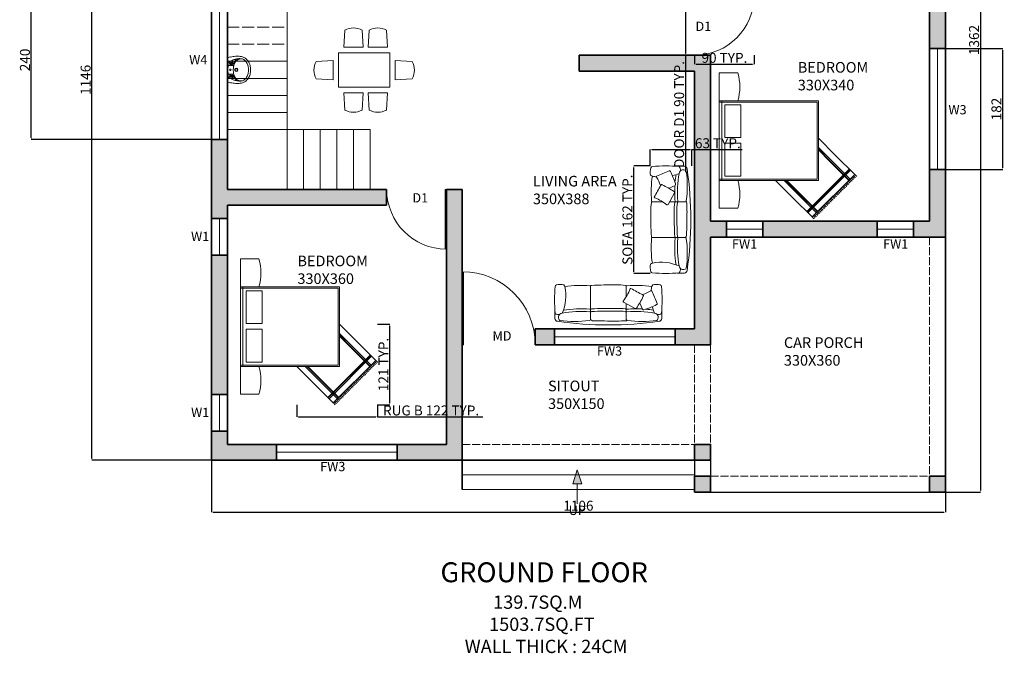
# Model space of a CAD drawing. Units: centimetres. Extents: x 2449 to 7478, y 778 to 2486.
# Tile 7 of 9: x 5994 to 7478, y 778 to 1732. Entities that reach past the tile are written whole.
import ezdxf

# ---------------------------------------------------------------- set-up
doc = ezdxf.new("R2010")
doc.units = ezdxf.units.CM
doc.linetypes.add('ACAD_ISO02W100', pattern=[15, 12, -3])
for name, color, linetype, lineweight in [('0.15', 34, 'Continuous', 15), ('A-ANNO-DIMS', 2, 'Continuous', 18), ('A-ANNO-SYMB', 8, 'Continuous', 18), ('A-ANNO-TEXT', 7, 'Continuous', 18), ('A-ANNO-TITL', 7, 'Continuous', 25), ('A-AREA-IDEN', 7, 'Continuous', 18), ('A-COLS', 7, 'Continuous', 35), ('A-COLS-PATT', 7, 'Continuous', 13), ('A-DOOR', 4, 'Continuous', 18), ('A-FLOR', 7, 'Continuous', 25), ('A-FLOR-FIXT', 8, 'Continuous', 18), ('A-FLOR-OVHD', 8, 'ACAD_ISO02W100', 18), ('A-FLOR-STRS', 7, 'Continuous', 18), ('A-FLOR-STRS-OVHD', 7, 'ACAD_ISO02W100', 13), ('A-WALL', 7, 'Continuous', 35), ('A-WALL-PATT', 7, 'Continuous', 13), ('B-FURNITURE', 22, 'Continuous', 18), ('Win', 1, 'Continuous', 18)]:
    doc.layers.add(name, color=color, linetype=linetype, lineweight=lineweight)
doc.styles.get("Standard").update_dxf_attribs({"font": 'arial.ttf'})
doc.dimstyles.new('ISO-25', dxfattribs={"dimtxt": 15, "dimasz": 2.5, "dimexe": 0, "dimexo": 0, "dimgap": 0, "dimtad": 1, "dimtxsty": 'Standard', "dimcen": 2.5, "dimadec": 0, "dimazin": 0, "dimtfac": 1, "dimtmove": 0, "dimatfit": 3, "dimfxl": 1, "dimarcsym": 0})

# ---------------------------------------------------------------- blocks, each defined once
blk = doc.blocks.new('ролар')
at = {"layer": 'B-FURNITURE'}
for p, q in [((182149, -12928), (182149, -13090)), ((182946, -12908), (182946, -13070)), ((183742, -12908), (183742, -13070)), ((184538, -12927), (184538, -13090)), ((182946, -13070), (182946, -13655)), ((183742, -13070), (183742, -13261)), ((183742, -13412), (183742, -13655))]:
    blk.add_line(p, q, dxfattribs=at)
blk.add_lwpolyline([(184124, -13426, 0.039108), (183972, -13160, 0.352413), (183942, -13151), (183685, -13293, 0.370087), (183675, -13320, -0.085318), (183831, -13592, 0.338149), (183848, -13604, -0.006963), (184118, -13456, 0.478074)], format="xyb", close=True, dxfattribs=at)
blk.add_lwpolyline([(184112, -13464, -0.054969), (184295, -13552, 0.338149), (184316, -13550, -0.006963), (184437, -13268, 0.478074), (184423, -13240, 0.039108), (184140, -13125, 0.352413), (184110, -13136), (184052, -13272)], format="xyb", dxfattribs=at)
for centre, radius, start, end in [((182209, -12928), 60, 90, 180), ((183344, -20690), 7904, 81.7476, 98.2524), ((182322, -12954), 95.7, 154.4132, 226.8965), ((182264, -12914), 28.1, 104.7154, 176.7534), ((182585, -15161), 2298, 81.7903, 98.2097), ((182918, -12915), 28.9, 15.2961, 99.1888), ((182999, -12942), 63.3, 99.7658, 147.0241), ((181568, 80195), 93085, 270.87421, 271.20678), ((183296, -20822), 7955, 86.6979, 88.3256), ((183770, -12915), 28.9, 80.8112, 164.7039), ((184102, -15161), 2298, 81.7903, 98.2097), ((184423, -12914), 28.1, 3.2466, 75.2846), ((184365, -12954), 95.7, 313.1035, 25.5868), ((184478, -12928), 60, 358.6006, 89.9879), ((186046, -13346), 3905, 175.5762, 184.4238), ((182224, -13128), 110, 72.3508, 130.321), ((182340, -12922), 131, 230.7956, 255.727), ((181452, -13440), 941, 347.608, 24.5904), ((182727, -10699), 2387, 259.8888, 274.8671), ((182725, -10712), 2434, 260.7796, 274.8194), ((182927, -13057), 20.3, 275.8765, 1.8), ((182927, -13117), 20.3, 275.8765, 1.8), ((182962, -13065), 17.3, 149.88, 272.0041), ((182962, -13125), 17.3, 149.88, 272.0041), ((183401, -6361), 6736, 266.2761, 271.089), ((183401, -6421), 6736, 266.2761, 271.089), ((183573, -12278), 819, 266.8813, 280.6931), ((183573, -12338), 819, 266.8813, 280.6931), ((183725, -13065), 17.3, 267.9959, 30.12), ((183725, -13125), 17.3, 267.9959, 30.12), ((183760, -13057), 20.3, 178.2, 264.1235), ((183760, -13117), 20.3, 178.2, 264.1235), ((183961, -10699), 2387, 265.1329, 280.1112), ((184001, -9721), 3425, 265.9379, 271.7664), ((184034, -11509), 1637, 275.2593, 281.2487), ((185235, -13440), 941, 155.4096, 164.8885), ((184348, -12922), 131, 284.273, 309.2044), ((184464, -13128), 110, 49.679, 107.6492), ((180641, -13346), 3905, 355.5762, 4.4238), ((182195, -13642), 42.7, 187.075, 250.1971), ((181903, -13435), 512, 330.8359, 336.0732), ((182722, -11168), 2503, 261.8987, 274.7524), ((182927, -13643), 20.3, 275.8765, 1.8), ((182962, -13651), 17.3, 149.88, 272.0041), ((183725, -13651), 17.3, 267.9959, 30.12), ((183760, -13643), 20.3, 178.2, 264.1235), ((183966, -11168), 2503, 265.2476, 278.1013), ((185235, -13440), 941, 186.9661, 192.392), ((184785, -13435), 512, 203.9268, 209.1641), ((184493, -13642), 42.7, 289.8029, 352.925), ((182270, -13358), 336, 254.5718, 283.8571), ((183401, -6946), 6736, 266.2761, 271.089), ((183573, -12863), 819, 266.8813, 280.6931), ((184418, -13358), 336, 256.1429, 285.4282)]:
    blk.add_arc(centre, radius, start, end, dxfattribs=at)
blk = doc.blocks.new('table-11')
at = {"color": 0, "linetype": 'ByBlock'}
for p, q in [((-1.122, 0.533), (-1.144, 0.134)), ((-0.716, 0.533), (-0.694, 0.134)), ((-0.554, 0.533), (-0.576, 0.134)), ((-0.148, 0.533), (-0.126, 0.134)), ((0, 0), (-1.2, 0)), ((-1.2, -0.8), (-1.2, 0)), ((-1.144, 0.134), (-0.694, 0.134)), ((-0.576, 0.134), (-0.126, 0.134)), ((0, -0.8), (0, 0)), ((-1.723, -0.197), (-1.324, -0.175)), ((-1.324, -0.625), (-1.324, -0.175)), ((0.523, -0.197), (0.124, -0.175)), ((0.124, -0.625), (0.124, -0.175)), ((-1.723, -0.603), (-1.324, -0.625)), ((0.523, -0.603), (0.124, -0.625)), ((0, -0.8), (-1.2, -0.8)), ((-1.144, -0.934), (-0.694, -0.934)), ((-1.122, -1.333), (-1.144, -0.934)), ((-0.716, -1.333), (-0.694, -0.934)), ((-0.576, -0.934), (-0.126, -0.934)), ((-0.554, -1.333), (-0.576, -0.934)), ((-0.148, -1.333), (-0.126, -0.934))]:
    blk.add_line(p, q, dxfattribs=at)
for centre, start, end in [((-0.919, 0.159), 61.4891, 118.5109), ((-0.351, 0.159), 61.4891, 118.5109), ((-1.349, -0.4), 151.4891, 208.5109), ((0.149, -0.4), 331.4891, 28.5109), ((-0.919, -0.959), 241.4891, 298.5109), ((-0.351, -0.959), 241.4891, 298.5109)]:
    blk.add_arc(centre, 0.425, start, end, dxfattribs=at)
blk = doc.blocks.new('A$C376C2187')
at = {"layer": 'B-FURNITURE'}
for p, q in [((-1.53, 1.82), (-1.53, 2.24)), ((-1.53, 2.24), (-0.9, 2.24)), ((-0.9, 0), (-0.9, 2.24)), ((-0.9, 2.24), (0.9, 2.24)), ((-0.9, 2.24), (-0.9, 1.82)), ((-0.87, 0.03), (-0.87, 2.24)), ((0.87, 2.24), (0.87, 0.03)), ((0.9, 2.24), (0.9, 0)), ((0.9, 1.82), (0.9, 2.24)), ((0.9, 2.24), (1.53, 2.24)), ((1.53, 2.24), (1.53, 1.82)), ((-0.9, 2.182), (0.9, 2.182)), ((-0.807, 2.112), (-0.057, 2.112)), ((-0.807, 1.749), (-0.807, 2.112)), ((-0.057, 2.112), (-0.057, 1.749)), ((0.069, 2.112), (0.807, 2.112)), ((0.069, 2.112), (0.069, 1.749)), ((0.807, 2.112), (0.807, 1.749)), ((-0.807, 1.749), (-0.057, 1.749)), ((0.069, 1.749), (0.807, 1.749)), ((0.9, 0), (-0.9, 0)), ((0.87, 0.03), (-0.87, 0.03))]:
    blk.add_line(p, q, dxfattribs=at)
for centre in [(-1.215, 2.926), (1.215, 2.926)]:
    blk.add_arc(centre, 1.15, 254.0965, 285.9035, dxfattribs=at)
blk = doc.blocks.new('lavamanos 2')
at = {"layer": '0.15'}
for p, q in [((0, 0.234), (0, -0.234)), ((-0.13, 0.11), (-0.131, 0.11)), ((-0.014, 0.087), (-0.13, 0.086)), ((-0.113, 0.112), (-0.107, 0.158)), ((-0.104, 0.111), (-0.098, 0.157)), ((-0.086, 0.109), (-0.081, 0.147)), ((-0.077, 0.107), (-0.072, 0.145)), ((-0.059, 0.105), (-0.055, 0.135)), ((-0.05, 0.104), (-0.046, 0.134)), ((-0.13, -0.11), (-0.131, -0.11)), ((-0.014, -0.087), (-0.13, -0.086)), ((-0.113, -0.112), (-0.107, -0.158)), ((-0.104, -0.111), (-0.098, -0.157)), ((-0.086, -0.109), (-0.081, -0.147)), ((-0.077, -0.107), (-0.072, -0.145)), ((-0.059, -0.105), (-0.055, -0.135)), ((-0.05, -0.104), (-0.046, -0.134))]:
    blk.add_line(p, q, dxfattribs=at)
for centre, radius in [((-0.178, 0), 0.035), ((-0.178, 0), 0.0235), ((-0.06, 0), 0.015)]:
    blk.add_circle(centre, radius, dxfattribs=at)
for centre, radius, start, end in [((-0.166, 0.001), 0.302, 136.5719, 154.3277), ((-0.242, 0.066), 0.202, 108.1945, 135.3686), ((-0.242, 0.065), 0.164, 121.9929, 150.5889), ((-0.266, 0.104), 0.119, 92.4774, 122.1411), ((-0.203, -0.086), 0.359, 91.203, 106.4255), ((-0.277, 0.068), 0.153, 57.2491, 95.54), ((-0.244, -0.013), 0.237, 77.2482, 96.4632), ((-0.221, -0.685), 0.959, 86.5514, 89.4131), ((-0.277, 0.068), 0.168, 56.8766, 64.9971), ((-0.222, 0.003), 0.218, 71.9849, 82.0124), ((-0.366, -0.002), 0.278, 40.3525, 49.2255), ((-0.212, -0.548), 0.82, 83.1224, 86.5796), ((-0.31, -0.315), 0.547, 69.5191, 73.4912), ((-0.299, -0.285), 0.516, 65.23, 69.5378), ((5.828, 30.215), 30.532, 258.7782, 258.876), ((-0.126, -0.066), 0.329, 69.0601, 78.8218), ((-0.02, 0.212), 0.0314, 54.7949, 69.0601), ((-0.005, 0.234), 0.005, 0, 54.7949), ((-0.209, 0.006), 0.256, 171.3102, 181.2627), ((-0.209, -0.006), 0.256, 178.7373, 188.6898), ((-0.056, -0.018), 0.411, 158.7011, 171.3102), ((0.466, -0.083), 0.895, 169.8632, 174.658), ((0.466, 0.083), 0.895, 185.342, 190.1368), ((-0.2, 0.026), 0.22, 147.1156, 167.4425), ((-0.366, -0.002), 0.263, 40.3525, 49.0046), ((-0.237, 0.11), 0.0921, 27.3186, 39.1156), ((-0.349, 0.036), 0.226, 22.3361, 30.8927), ((-0.237, 0.11), 0.107, 27.5743, 39.1156), ((-0.349, 0.036), 0.241, 22.1921, 30.7838), ((-1.266, -0.239), 1.182, 16.3631, 17.7767), ((-0.132, 0.117), 0.007, 197.4099, 270.4949), ((0.185, 0.165), 0.325, 192.5389, 196.7072), ((-0.13, 0.117), 0.007, 270.4949, 17.3953), ((-1.266, -0.239), 1.197, 17.3953, 17.8049), ((0.389, 0.121), 0.517, 185.5053, 189.8131), ((-0.718, -0.007), 0.599, 0.6765, 3.8216), ((-0.718, 0.007), 0.599, 356.1784, 359.3235), ((-0.108, 0.111), 0.0045, 172.614, 352.614), ((-0.102, 0.158), 0.0045, 352.614, 172.614), ((-0.081, 0.108), 0.0045, 172.614, 352.614), ((-0.278, -0.241), 0.466, 60.2413, 65.2382), ((-0.076, 0.146), 0.0045, 352.614, 172.614), ((-0.054, 0.104), 0.0045, 172.614, 352.614), ((-0.05, 0.135), 0.0045, 352.614, 172.614), ((-0.065, 0.118), 0.049, 1.5827, 68.6208), ((-2.148, 0.001), 2.135, 359.9754, 3.1901), ((-2.148, -0.001), 2.135, 356.8099, 0.0246), ((-0.056, 0.018), 0.411, 188.6898, 201.2989), ((-0.166, -0.001), 0.302, 205.6723, 223.4281), ((-0.2, -0.026), 0.22, 192.5575, 212.8844), ((-0.242, -0.065), 0.164, 209.4111, 238.0071), ((-0.277, -0.068), 0.153, 264.46, 302.7509), ((-0.366, 0.002), 0.263, 310.9954, 319.6475), ((-0.366, 0.002), 0.278, 310.7745, 319.6475), ((-0.237, -0.11), 0.0921, 320.8844, 332.6814), ((-0.349, -0.036), 0.226, 329.1073, 337.6639), ((-0.237, -0.11), 0.107, 320.8844, 332.4257), ((-0.349, -0.036), 0.241, 329.2162, 337.8079), ((-1.266, 0.239), 1.182, 342.2233, 343.6369), ((-0.132, -0.117), 0.007, 89.5051, 162.5901), ((0.185, -0.165), 0.325, 163.2928, 167.4611), ((-0.13, -0.117), 0.007, 342.6047, 89.5051), ((0.389, -0.121), 0.517, 170.1869, 174.4947), ((-1.266, 0.239), 1.197, 342.1951, 342.6047), ((-0.299, 0.286), 0.516, 290.4622, 294.77), ((-0.108, -0.111), 0.0045, 7.386, 187.386), ((-0.102, -0.158), 0.0045, 187.386, 7.386), ((-0.081, -0.108), 0.0045, 7.386, 187.386), ((-0.278, 0.241), 0.466, 294.7618, 299.7587), ((-0.076, -0.146), 0.0045, 187.386, 7.386), ((-0.054, -0.104), 0.0045, 7.386, 187.386), ((-0.05, -0.135), 0.0045, 187.386, 7.386), ((-0.065, -0.118), 0.049, 291.3792, 358.4173), ((-0.242, -0.066), 0.202, 224.6314, 251.8055), ((-0.266, -0.104), 0.119, 237.8589, 267.5226), ((-0.203, 0.086), 0.359, 253.5745, 268.797), ((-0.244, 0.013), 0.237, 263.5368, 282.7518), ((-0.221, 0.685), 0.959, 270.5869, 273.4486), ((-0.277, -0.068), 0.168, 295.0029, 303.1234), ((-0.222, -0.003), 0.218, 277.9876, 288.0151), ((-0.212, 0.548), 0.82, 273.4204, 276.8776), ((-0.31, 0.315), 0.547, 286.5088, 290.4809), ((5.828, -30.215), 30.532, 101.124, 101.2218), ((-0.126, 0.066), 0.329, 281.1782, 290.9399), ((-0.02, -0.212), 0.0314, 290.9399, 305.2051), ((-0.005, -0.234), 0.005, 305.2051, 0)]:
    blk.add_arc(centre, radius, start, end, dxfattribs=at)
blk = doc.blocks.new('1')
for p, q in [((5854.1, 1703.8), (5854.1, 1593.8)), ((5856.1, 1703.8), (5856.1, 1593.8)), ((5856.1, 1593.8), (5854.1, 1593.8))]:
    blk.add_line(p, q)
blk.add_arc((5854.1, 1593.8), 110, 0, 90)
blk = doc.blocks.new('2')
for p, q in [((5717.3, 1812.7), (5717.3, 1722.7)), ((5719.3, 1812.7), (5719.3, 1722.7)), ((5719.3, 1722.7), (5717.3, 1722.7))]:
    blk.add_line(p, q)
blk.add_arc((5717.3, 1722.7), 90, 0, 90)
blk = doc.blocks.new('*D64')
at = {"layer": 'A-ANNO-DIMS', "color": 0, "lineweight": -2, "transparency": 16777216}
for p, q in [((7389, 2382.3), (7441.8, 2382.3)), ((7441.8, 2379.8), (7441.8, 1022.8)), ((7389, 1020.3), (7441.8, 1020.3))]:
    blk.add_line(p, q, dxfattribs=at)
at = {"layer": 'A-ANNO-DIMS', "color": 0, "transparency": 16777216}
for points in [[(7441.4, 2379.8), (7442.2, 2379.8), (7441.8, 2382.3)], [(7441.4, 1022.8), (7442.2, 1022.8), (7441.8, 1020.3)]]:
    blk.add_solid(points, dxfattribs=at)
at = {"layer": 'Defpoints', "color": 0, "transparency": 16777216}
for p in [(7389, 2382.3), (7389, 1020.3), (7441.8, 1020.3)]:
    blk.add_point(p, dxfattribs=at)
at = {"layer": 'A-ANNO-DIMS', "color": 0, "transparency": 16777216, "insert": (7434.1, 1701.3), "char_height": 15, "attachment_point": 5, "rotation": 90}
blk.add_mtext('1362', dxfattribs=at)
blk = doc.blocks.new('*D65')
at = {"layer": 'A-ANNO-DIMS', "color": 0, "lineweight": -2, "transparency": 16777216}
for p, q in [((6283, 1068.3), (6283, 990.3)), ((7389, 1020.3), (7389, 990.3)), ((6285.5, 990.3), (7386.5, 990.3))]:
    blk.add_line(p, q, dxfattribs=at)
at = {"layer": 'A-ANNO-DIMS', "color": 0, "transparency": 16777216}
for points in [[(6285.5, 990.7), (6285.5, 989.9), (6283, 990.3)], [(7386.5, 990.7), (7386.5, 989.9), (7389, 990.3)]]:
    blk.add_solid(points, dxfattribs=at)
at = {"layer": 'Defpoints', "color": 0, "transparency": 16777216}
for p in [(6283, 1068.3), (7389, 1020.3), (7389, 990.3)]:
    blk.add_point(p, dxfattribs=at)
at = {"layer": 'A-ANNO-DIMS', "color": 0, "transparency": 16777216, "insert": (6836, 998), "char_height": 15, "attachment_point": 5}
blk.add_mtext('1106', dxfattribs=at)
blk = doc.blocks.new('*D66')
at = {"layer": 'A-ANNO-DIMS', "color": 0, "lineweight": -2, "transparency": 16777216}
for p, q in [((6155, 2214.3), (6103, 2214.3)), ((6103, 1070.8), (6103, 2211.8)), ((6283, 1068.3), (6103, 1068.3))]:
    blk.add_line(p, q, dxfattribs=at)
at = {"layer": 'A-ANNO-DIMS', "color": 0, "transparency": 16777216}
for points in [[(6102.6, 2211.8), (6103.4, 2211.8), (6103, 2214.3)], [(6102.6, 1070.8), (6103.4, 1070.8), (6103, 1068.3)]]:
    blk.add_solid(points, dxfattribs=at)
at = {"layer": 'Defpoints', "color": 0, "transparency": 16777216}
for p in [(6103, 2214.3), (6155, 2214.3), (6283, 1068.3)]:
    blk.add_point(p, dxfattribs=at)
at = {"layer": 'A-ANNO-DIMS', "color": 0, "transparency": 16777216, "insert": (6095.4, 1641.3), "char_height": 15, "attachment_point": 5, "rotation": 90}
blk.add_mtext('1146', dxfattribs=at)
blk = doc.blocks.new('RUG-FRINGED-B')
for p, q in [((90.4, 95.2), (64.4, 121.3)), ((64.4, 107.4), (83.5, 88.3)), ((64.4, 104.7), (82.1, 86.9)), ((64.4, 103.6), (81.6, 86.3)), ((90.4, 95.2), (119.1, 66.6)), ((110.7, 74.9), (46.8, 11)), ((111.3, 74.4), (47.4, 10.4)), ((110.2, 57.7), (81.6, 86.3)), ((110.8, 58.3), (82.1, 86.9)), ((112.1, 59.7), (83.5, 88.3)), ((112.7, 73), (48.7, 9)), ((119.1, 66.6), (55.1, 2.7)), ((112.3, 59.9), (115, 57.3)), ((114, 61.6), (116.6, 58.9)), ((115.7, 63.2), (118.3, 60.6)), ((117.4, 64.9), (120, 62.3)), ((119.1, 66.6), (121.7, 64)), ((0, 57.8), (26.5, 31.3)), ((32.9, 37.7), (12.8, 57.8)), ((34.2, 39), (15.5, 57.8)), ((34.8, 39.6), (16.7, 57.8)), ((97.2, 44.8), (99.8, 42.1)), ((98.9, 46.4), (101.5, 43.8)), ((100.6, 48.1), (103.2, 45.5)), ((102.3, 49.8), (104.9, 47.2)), ((103.9, 51.5), (106.6, 48.9)), ((105.6, 53.2), (108.2, 50.5)), ((107.3, 54.8), (109.9, 52.2)), ((109, 56.5), (111.6, 53.9)), ((110.7, 58.2), (113.3, 55.6)), ((55.1, 2.7), (26.5, 31.3)), ((32.9, 37.7), (61.5, 9)), ((34.2, 39), (62.9, 10.4)), ((34.8, 39.6), (63.4, 11)), ((83.8, 31.3), (86.4, 28.7)), ((85.5, 33), (88.1, 30.4)), ((87.1, 34.7), (89.8, 32.1)), ((88.8, 36.4), (91.4, 33.7)), ((90.5, 38), (93.1, 35.4)), ((92.2, 39.7), (94.8, 37.1)), ((93.9, 41.4), (96.5, 38.8)), ((95.5, 43.1), (98.2, 40.5)), ((68.7, 16.2), (71.3, 13.6)), ((70.3, 17.9), (73, 15.3)), ((72, 19.6), (74.6, 16.9)), ((73.7, 21.2), (76.3, 18.6)), ((75.4, 22.9), (78, 20.3)), ((77.1, 24.6), (79.7, 22)), ((78.7, 26.3), (81.4, 23.7)), ((80.4, 28), (83, 25.3)), ((82.1, 29.6), (84.7, 27)), ((55.2, 2.8), (57.8, 0.1)), ((56.9, 4.4), (59.5, 1.8)), ((58.6, 6.1), (61.2, 3.5)), ((60.3, 7.8), (62.9, 5.2)), ((61.9, 9.5), (64.6, 6.9)), ((63.6, 11.2), (66.2, 8.5)), ((65.3, 12.8), (67.9, 10.2)), ((67, 14.5), (69.6, 11.9))]:
    blk.add_line(p, q)
for centre in [(118.4, 60.6), (120.1, 62.2), (121.8, 63.9), (103.3, 45.4), (105, 47.1), (106.6, 48.8), (108.3, 50.5), (110, 52.2), (111.7, 53.8), (113.4, 55.5), (115, 57.2), (116.7, 58.9), (88.1, 30.3), (89.8, 32), (91.5, 33.7), (93.2, 35.4), (94.9, 37), (96.5, 38.7), (98.2, 40.4), (99.9, 42.1), (101.6, 43.8), (73, 15.2), (74.7, 16.9), (76.4, 18.6), (78.1, 20.2), (79.7, 21.9), (81.4, 23.6), (83.1, 25.3), (84.8, 27), (86.5, 28.6), (57.9, 0.1), (59.6, 1.8), (61.3, 3.4), (62.9, 5.1), (64.6, 6.8), (66.3, 8.5), (68, 10.2), (69.7, 11.8), (71.3, 13.5)]:
    blk.add_circle(centre, 0.0789)
blk = doc.blocks.new('ARROW-ENTRY-UP')
at = {"transparency": 33554687}
h = blk.add_hatch(color=256, dxfattribs=at)
h.dxf.hatch_style = 1
h.paths.add_polyline_path([(-6.8, 30.3), (6.8, 30.3), (0, 51.2)])
blk.add_line((0, 30.3), (0, 0))
blk.add_lwpolyline([(0, 51.2), (-6.8, 30.3), (6.8, 30.3)], close=True)
blk = doc.blocks.new('*D74')
at = {"layer": 'A-ANNO-DIMS', "color": 0, "lineweight": -2, "transparency": 16777216}
for p, q in [((7011, 1768.3), (6997.5, 1768.3)), ((6997.5, 1765.8), (6997.5, 1680.8)), ((7011, 1678.3), (6997.5, 1678.3)), ((6997.5, 1678.3), (6997.5, 1502.3))]:
    blk.add_line(p, q, dxfattribs=at)
at = {"layer": 'A-ANNO-DIMS', "color": 0, "transparency": 16777216}
for points in [[(6997.1, 1765.8), (6997.9, 1765.8), (6997.5, 1768.3)], [(6997.1, 1680.8), (6997.9, 1680.8), (6997.5, 1678.3)]]:
    blk.add_solid(points, dxfattribs=at)
at = {"layer": 'Defpoints', "color": 0, "transparency": 16777216}
for p in [(7011, 1768.3), (6997.5, 1678.3), (7011, 1678.3)]:
    blk.add_point(p, dxfattribs=at)
at = {"layer": 'A-ANNO-DIMS', "color": 0, "transparency": 16777216, "insert": (6989.7, 1589.1), "char_height": 15, "attachment_point": 5, "rotation": 90}
blk.add_mtext('DOOR D1 90 TYP.', dxfattribs=at)
blk = doc.blocks.new('*D75')
at = {"layer": 'A-ANNO-DIMS', "color": 0, "lineweight": -2, "transparency": 16777216}
for p, q in [((7011, 1678.3), (7011, 1664.8)), ((7101, 1678.3), (7101, 1664.8)), ((7013.5, 1664.8), (7098.5, 1664.8))]:
    blk.add_line(p, q, dxfattribs=at)
at = {"layer": 'A-ANNO-DIMS', "color": 0, "transparency": 16777216}
for points in [[(7013.5, 1665.3), (7013.5, 1664.4), (7011, 1664.8)], [(7098.5, 1665.3), (7098.5, 1664.4), (7101, 1664.8)]]:
    blk.add_solid(points, dxfattribs=at)
at = {"layer": 'Defpoints', "color": 0, "transparency": 16777216}
for p in [(7011, 1678.3), (7101, 1678.3), (7101, 1664.8)]:
    blk.add_point(p, dxfattribs=at)
at = {"layer": 'A-ANNO-DIMS', "color": 0, "transparency": 16777216, "insert": (7056, 1672.5), "char_height": 15, "attachment_point": 5}
blk.add_mtext('90 TYP.', dxfattribs=at)
blk = doc.blocks.new('*D82')
at = {"layer": 'A-ANNO-DIMS', "color": 0, "lineweight": -2, "transparency": 16777216}
for p, q in [((6943.9, 1511.9), (6919.5, 1511.9)), ((6919.5, 1351.9), (6919.5, 1509.4)), ((6943.9, 1349.4), (6919.5, 1349.4))]:
    blk.add_line(p, q, dxfattribs=at)
at = {"layer": 'A-ANNO-DIMS', "color": 0, "transparency": 16777216}
for points in [[(6919.1, 1509.4), (6919.9, 1509.4), (6919.5, 1511.9)], [(6919.1, 1351.9), (6919.9, 1351.9), (6919.5, 1349.4)]]:
    blk.add_solid(points, dxfattribs=at)
at = {"layer": 'Defpoints', "color": 0, "transparency": 16777216}
for p in [(6919.5, 1511.9), (6943.9, 1511.9), (6943.9, 1349.4)]:
    blk.add_point(p, dxfattribs=at)
at = {"layer": 'A-ANNO-DIMS', "color": 0, "transparency": 16777216, "insert": (6911.8, 1430.7), "char_height": 15, "attachment_point": 5, "rotation": 90}
blk.add_mtext('SOFA 162 TYP.', dxfattribs=at)
blk = doc.blocks.new('*D83')
at = {"layer": 'A-ANNO-DIMS', "color": 0, "lineweight": -2, "transparency": 16777216}
for p, q in [((6943.9, 1511.9), (6943.9, 1536.3)), ((6946.4, 1536.3), (7004.6, 1536.3)), ((7007.1, 1511.9), (7007.1, 1536.3)), ((7007.1, 1536.3), (7082.7, 1536.3))]:
    blk.add_line(p, q, dxfattribs=at)
at = {"layer": 'A-ANNO-DIMS', "color": 0, "transparency": 16777216}
for points in [[(6946.4, 1536.7), (6946.4, 1535.9), (6943.9, 1536.3)], [(7004.6, 1536.7), (7004.6, 1535.9), (7007.1, 1536.3)]]:
    blk.add_solid(points, dxfattribs=at)
at = {"layer": 'Defpoints', "color": 0, "transparency": 16777216}
for p in [(7007.1, 1536.3), (6943.9, 1511.9), (7007.1, 1511.9)]:
    blk.add_point(p, dxfattribs=at)
at = {"layer": 'A-ANNO-DIMS', "color": 0, "transparency": 16777216, "insert": (7046.1, 1543.9), "char_height": 15, "attachment_point": 5}
blk.add_mtext('63 TYP.', dxfattribs=at)
blk = doc.blocks.new('*D84')
at = {"layer": 'A-ANNO-DIMS', "color": 0, "lineweight": -2, "transparency": 16777216}
for p, q in [((6411.6, 1151.9), (6411.6, 1133.6)), ((6533.4, 1151.9), (6533.4, 1133.6)), ((6414.1, 1133.6), (6530.9, 1133.6)), ((6533.4, 1133.6), (6692, 1133.6))]:
    blk.add_line(p, q, dxfattribs=at)
at = {"layer": 'A-ANNO-DIMS', "color": 0, "transparency": 16777216}
for points in [[(6414.1, 1134), (6414.1, 1133.2), (6411.6, 1133.6)], [(6530.9, 1134), (6530.9, 1133.2), (6533.4, 1133.6)]]:
    blk.add_solid(points, dxfattribs=at)
at = {"layer": 'Defpoints', "color": 0, "transparency": 16777216}
for p in [(6411.6, 1151.9), (6533.4, 1151.9), (6533.4, 1133.6)]:
    blk.add_point(p, dxfattribs=at)
at = {"layer": 'A-ANNO-DIMS', "color": 0, "transparency": 16777216, "insert": (6614, 1141.4), "char_height": 15, "attachment_point": 5}
blk.add_mtext('RUG B 122 TYP.', dxfattribs=at)
blk = doc.blocks.new('*D85')
at = {"layer": 'A-ANNO-DIMS', "color": 0, "lineweight": -2, "transparency": 16777216}
for p, q in [((6533.4, 1273.2), (6551.7, 1273.2)), ((6551.7, 1154.4), (6551.7, 1270.7)), ((6533.4, 1151.9), (6551.7, 1151.9))]:
    blk.add_line(p, q, dxfattribs=at)
at = {"layer": 'A-ANNO-DIMS', "color": 0, "transparency": 16777216}
for points in [[(6551.3, 1270.7), (6552.1, 1270.7), (6551.7, 1273.2)], [(6551.3, 1154.4), (6552.1, 1154.4), (6551.7, 1151.9)]]:
    blk.add_solid(points, dxfattribs=at)
at = {"layer": 'Defpoints', "color": 0, "transparency": 16777216}
for p in [(6533.4, 1273.2), (6551.7, 1273.2), (6533.4, 1151.9)]:
    blk.add_point(p, dxfattribs=at)
at = {"layer": 'A-ANNO-DIMS', "color": 0, "transparency": 16777216, "insert": (6544.2, 1212.6), "char_height": 15, "attachment_point": 5, "rotation": 90}
blk.add_mtext('121 TYP.', dxfattribs=at)
blk = doc.blocks.new('*D114')
at = {"layer": 'A-ANNO-DIMS', "color": 0, "lineweight": -2, "transparency": 16777216}
for p, q in [((7389, 1688.3), (7475.5, 1688.3)), ((7475.5, 1508.8), (7475.5, 1685.8)), ((7389, 1506.3), (7475.5, 1506.3))]:
    blk.add_line(p, q, dxfattribs=at)
at = {"layer": 'A-ANNO-DIMS', "color": 0, "transparency": 16777216}
for points in [[(7475.1, 1685.8), (7475.9, 1685.8), (7475.5, 1688.3)], [(7475.1, 1508.8), (7475.9, 1508.8), (7475.5, 1506.3)]]:
    blk.add_solid(points, dxfattribs=at)
at = {"layer": 'Defpoints', "color": 0, "transparency": 16777216}
for p in [(7389, 1688.3), (7475.5, 1688.3), (7389, 1506.3)]:
    blk.add_point(p, dxfattribs=at)
at = {"layer": 'A-ANNO-DIMS', "color": 0, "transparency": 16777216, "insert": (7467.8, 1597.3), "char_height": 15, "attachment_point": 5, "rotation": 90}
blk.add_mtext('182', dxfattribs=at)
blk = doc.blocks.new('*D115')
at = {"layer": 'A-ANNO-DIMS', "color": 0, "lineweight": -2, "transparency": 16777216}
for p, q in [((6283, 1791.3), (6011.6, 1791.3)), ((6011.6, 1553.8), (6011.6, 1788.8)), ((6283, 1551.3), (6011.6, 1551.3))]:
    blk.add_line(p, q, dxfattribs=at)
at = {"layer": 'A-ANNO-DIMS', "color": 0, "transparency": 16777216}
for points in [[(6011.2, 1788.8), (6012.1, 1788.8), (6011.6, 1791.3)], [(6011.2, 1553.8), (6012.1, 1553.8), (6011.6, 1551.3)]]:
    blk.add_solid(points, dxfattribs=at)
at = {"layer": 'Defpoints', "color": 0, "transparency": 16777216}
for p in [(6011.6, 1791.3), (6283, 1791.3), (6283, 1551.3)]:
    blk.add_point(p, dxfattribs=at)
at = {"layer": 'A-ANNO-DIMS', "color": 0, "transparency": 16777216, "insert": (6004, 1671.3), "char_height": 15, "attachment_point": 5, "rotation": 90}
blk.add_mtext('240', dxfattribs=at)

msp = doc.modelspace()

# ---------------------------------------------------------------- hatches: boundary and pattern name
at = {"layer": 'A-COLS-PATT'}
h = msp.add_hatch(color=256, dxfattribs=at)
h.dxf.hatch_style = 1
h.paths.add_polyline_path([(7035.006, 1092.34), (7011.006, 1092.34), (7011.006, 1068.34), (7035.006, 1068.34)])
h = msp.add_hatch(color=256, dxfattribs=at)
h.dxf.hatch_style = 1
h.paths.add_polyline_path([(7011.006, 1020.34), (7035.006, 1020.34), (7035.006, 1044.34), (7011.006, 1044.34)])
h = msp.add_hatch(color=256, dxfattribs=at)
h.dxf.hatch_style = 1
h.paths.add_polyline_path([(7365.006, 1020.34), (7389.006, 1020.34), (7389.006, 1044.34), (7365.006, 1044.34)])
at = {"layer": 'A-WALL-PATT'}
h = msp.add_hatch(color=256, dxfattribs=at)
h.dxf.hatch_style = 1
h.paths.add_polyline_path([(6637.006, 1092.34), (6563.006, 1092.34), (6563.006, 1068.34), (6661.006, 1068.34), (6661.006, 1476.34), (6637.006, 1476.34)])
h.paths.add_polyline_path([(6283.006, 1167.34), (6307.006, 1167.34), (6307.006, 1377.34), (6283.006, 1377.34)])
h.paths.add_polyline_path([(6381.006, 1068.34), (6381.006, 1092.34), (6307.006, 1092.34), (6307.006, 1112.34), (6283.006, 1112.34), (6283.006, 1068.34)])
h.paths.add_polyline_path([(6307.006, 1551.34), (6283.006, 1551.34), (6283.006, 1432.34), (6307.006, 1432.34), (6307.006, 1452.34), (6547.006, 1452.34), (6547.006, 1476.34), (6307.006, 1476.34)])
h.paths.add_polyline_path([(7011.006, 1654.34), (7011.006, 1266.34), (6982.006, 1266.34), (6982.006, 1242.34), (7035.006, 1242.34), (7035.006, 1404.34), (7059.006, 1404.34), (7059.006, 1428.34), (7035.006, 1428.34), (7035.006, 1678.34), (6837.006, 1678.34), (6837.006, 1654.34)])
h.paths.add_polyline_path([(6800.006, 1266.34), (6771.006, 1266.34), (6771.006, 1242.34), (6800.006, 1242.34)])
h.paths.add_polyline_path([(7389.006, 1506.339), (7365.006, 1506.339), (7365.006, 1428.34), (7341.006, 1428.34), (7341.006, 1404.34), (7389.006, 1404.34)])
h.paths.add_polyline_path([(7286.006, 1404.34), (7286.006, 1428.34), (7114.006, 1428.34), (7114.006, 1404.34)])
h.paths.add_polyline_path([(7365.006, 1688.339), (7389.006, 1688.339), (7389.006, 1826.34), (7365.006, 1826.34), (7365.006, 1792.34), (7224.006, 1792.34), (7224.006, 1768.34), (7365.006, 1768.34)])
h.paths.add_polyline_path([(7365.006, 1956.34), (7125.006, 1956.34), (7125.006, 1792.34), (7011.006, 1792.34), (7011.006, 1768.34), (7149.006, 1768.34), (7149.006, 1932.34), (7365.006, 1932.34), (7365.006, 1898.34), (7389.006, 1898.34), (7389.006, 2065.339), (7365.006, 2065.339)])
h.paths.add_polyline_path([(7365.006, 2358.34), (7365.006, 2247.339), (7389.006, 2247.339), (7389.006, 2382.34), (7341.006, 2382.34), (7341.006, 2358.34)])
h.paths.add_polyline_path([(7114.006, 2382.34), (7114.006, 2358.34), (7286.006, 2358.34), (7286.006, 2382.34)])
h.paths.add_polyline_path([(7035.006, 2358.34), (7059.006, 2358.34), (7059.006, 2382.34), (7011.006, 2382.34), (7011.006, 2214.34), (6972.006, 2214.34), (6972.006, 2190.34), (7011.006, 2190.34), (7011.006, 2065.34), (7035.006, 2065.34)])
h.paths.add_polyline_path([(6808.006, 2214.34), (6808.006, 2190.34), (6837.006, 2190.34), (6837.006, 1966.34), (7011.006, 1966.34), (7011.006, 1932.34), (7035.006, 1932.34), (7035.006, 1990.34), (6861.006, 1990.34), (6861.006, 2190.34), (6900.006, 2190.34), (6900.006, 2214.34)])
h.paths.add_polyline_path([(6707.006, 2190.34), (6736.006, 2190.34), (6736.006, 2214.34), (6609.006, 2214.34), (6609.006, 2190.34), (6683.006, 2190.34), (6683.006, 1836.34), (6707.006, 1836.34), (6707.006, 1966.34), (6762.006, 1966.34), (6762.006, 1990.34), (6707.006, 1990.34)])
h.paths.add_polyline_path([(6315.006, 2214.34), (6315.006, 2190.34), (6329.006, 2190.34), (6329.006, 1935.34), (6353.006, 1935.34), (6353.006, 2190.34), (6427.006, 2190.34), (6427.006, 2214.34)])
h.paths.add_polyline_path([(6155.006, 2152.839), (6179.006, 2152.839), (6179.006, 2190.34), (6193.006, 2190.34), (6193.006, 2214.34), (6155.006, 2214.34)])
h.paths.add_polyline_path([(6155.006, 1935.34), (6179.006, 1935.34), (6179.006, 1970.839), (6155.006, 1970.839)])
h.paths.add_polyline_path([(6283.006, 1836.34), (6283.006, 1791.34), (6307.006, 1791.34), (6307.006, 1836.34), (6593.006, 1836.34), (6593.006, 1860.34), (6155.006, 1860.34), (6155.006, 1836.34)])

# ---------------------------------------------------------------- linework, layer by layer
at = {"layer": 'A-COLS'}
for points in [[(7011.006, 1068.34), (7035.006, 1068.34), (7035.006, 1092.34), (7011.006, 1092.34)], [(7011.006, 1020.34), (7035.006, 1020.34), (7035.006, 1044.34), (7011.006, 1044.34)], [(7365.006, 1020.34), (7389.006, 1020.34), (7389.006, 1044.34), (7365.006, 1044.34)]]:
    msp.add_lwpolyline(points, close=True, dxfattribs=at)
at = {"layer": 'A-FLOR'}
for p, q in [((7011.006, 1092.34), (7011.006, 1020.34)), ((7035.006, 1092.34), (7035.006, 1044.34)), ((7011.006, 1044.34), (7035.006, 1044.34)), ((7011.006, 1020.34), (7389.006, 1020.34))]:
    msp.add_line(p, q, dxfattribs=at)
at = {"layer": 'A-FLOR-OVHD'}
for p, q in [((7365.006, 1404.34), (7365.006, 1044.34)), ((7011.006, 1242.34), (7011.006, 1092.34)), ((7035.006, 1242.34), (7035.006, 1092.34)), ((6661.006, 1092.34), (7035.006, 1092.34)), ((7035.006, 1044.34), (7365.006, 1044.34))]:
    msp.add_line(p, q, dxfattribs=at)
at = {"layer": 'A-FLOR-STRS'}
for p, q in [((6397.006, 1836.34), (6397.006, 1476.34)), ((6307.006, 1669.21), (6397.006, 1669.21)), ((6307.006, 1643.47), (6397.006, 1643.47)), ((6307.006, 1617.76), (6397.006, 1617.76)), ((6307.006, 1592.05), (6397.006, 1592.05)), ((6307.006, 1566.34), (6522.006, 1566.34)), ((6422.006, 1566.34), (6422.006, 1476.34)), ((6447.006, 1566.34), (6447.006, 1476.34)), ((6472.006, 1566.34), (6472.006, 1476.34)), ((6497.006, 1566.34), (6497.006, 1476.34)), ((6522.006, 1566.34), (6522.006, 1476.34)), ((6661.006, 1046.34), (7011.006, 1046.34)), ((6661.006, 1024.34), (7011.006, 1024.34))]:
    msp.add_line(p, q, dxfattribs=at)
at = {"layer": 'A-FLOR-STRS-OVHD', "ltscale": 1.5}
for p, q in [((6307.006, 1720.63), (6397.006, 1720.63)), ((6307.006, 1694.92), (6397.006, 1694.92))]:
    msp.add_line(p, q, dxfattribs=at)
at = {"layer": 'A-WALL'}
for p, q in [((7389.006, 2382.34), (7389.006, 1020.34)), ((6283.006, 1836.34), (6283.006, 1068.34)), ((6307.006, 1836.34), (6307.006, 1476.34)), ((7365.006, 1768.34), (7365.006, 1428.34)), ((6837.006, 1678.34), (6837.006, 1654.34)), ((6837.006, 1678.34), (7035.006, 1678.34)), ((7035.006, 1678.34), (7035.006, 1428.34)), ((7365.006, 1688.339), (7389.006, 1688.339)), ((6837.006, 1654.34), (7011.006, 1654.34)), ((7011.006, 1654.34), (7011.006, 1266.34)), ((6307.006, 1551.34), (6283.006, 1551.34)), ((7365.006, 1506.339), (7389.006, 1506.339)), ((6307.006, 1476.34), (6547.006, 1476.34)), ((6547.006, 1476.34), (6547.006, 1452.34)), ((6637.006, 1476.34), (6637.006, 1092.34)), ((6637.006, 1476.34), (6661.006, 1476.34)), ((6661.006, 1476.34), (6661.006, 1024.34)), ((6307.006, 1452.34), (6307.006, 1092.34)), ((6307.006, 1452.34), (6547.006, 1452.34)), ((6283.006, 1432.34), (6307.006, 1432.34)), ((7035.006, 1428.34), (7365.006, 1428.34)), ((7059.006, 1428.34), (7059.006, 1404.34)), ((7114.006, 1428.34), (7114.006, 1404.34)), ((7286.006, 1428.34), (7286.006, 1404.34)), ((7341.006, 1428.34), (7341.006, 1404.34)), ((7035.006, 1404.34), (7035.006, 1242.34)), ((7035.006, 1404.34), (7389.006, 1404.34)), ((6283.006, 1377.34), (6307.006, 1377.34)), ((6771.006, 1266.34), (6771.006, 1242.34)), ((6771.006, 1266.34), (7011.006, 1266.34)), ((6800.006, 1266.34), (6800.006, 1242.34)), ((6982.006, 1266.34), (6982.006, 1242.34)), ((6771.006, 1242.34), (7035.006, 1242.34)), ((6283.006, 1167.34), (6307.006, 1167.34)), ((6283.006, 1112.34), (6307.006, 1112.34)), ((6307.006, 1092.34), (6637.006, 1092.34)), ((6381.006, 1092.34), (6381.006, 1068.34)), ((6563.006, 1092.34), (6563.006, 1068.34)), ((6283.006, 1068.34), (7035.006, 1068.34))]:
    msp.add_line(p, q, dxfattribs=at)
at = {"layer": 'Win'}
for p, q in [((6295.006, 1791.34), (6295.006, 1551.34)), ((7377.006, 1688.339), (7377.006, 1506.339)), ((6295.006, 1432.34), (6295.006, 1377.34)), ((7059.006, 1416.34), (7114.006, 1416.34)), ((7286.006, 1416.34), (7341.006, 1416.34)), ((6800.006, 1254.34), (6982.006, 1254.34)), ((6295.006, 1112.34), (6295.006, 1167.34)), ((6381.006, 1080.34), (6563.006, 1080.34))]:
    msp.add_line(p, q, dxfattribs=at)

# ---------------------------------------------------------------- block references
at = {"layer": 'A-ANNO-SYMB'}
msp.add_blockref('ARROW-ENTRY-UP', (6834.279, 1002.514), dxfattribs=at)
at = {"layer": 'A-DOOR'}
for p, rotation in [((5288.291, 7485.689), 270), ((12354.355, 3199.054), 180)]:
    msp.add_blockref('2', p, dxfattribs=dict(at, rotation=rotation))
msp.add_blockref('1', (806.885, -351.413), dxfattribs=at)
at = {"layer": 'A-FLOR-FIXT', "xscale": 75.44223598555656, "yscale": 75.44223598555656, "zscale": 75.44223598555656, "rotation": 179.99990349049}
msp.add_blockref('lavamanos 2', (6307.006, 1656.34), dxfattribs=at)
at = {"layer": 'B-FURNITURE'}
for name, p, xscale, yscale, zscale, rotation in [('table-11', (6474.451, 1630.173), 64.48907140530227, 64.48907140530227, 64.48907140530227, 180), ('A$C376C2187', (7197.496, 1549.792), 66.63496932822166, 66.63496932822166, 66.63496932822166, 90), ('ролар', (7865.915, -10910.435), -0.0673113048210398, 0.0673113048210398, 0.0673113048210398, 270), ('A$C376C2187', (6475.954, 1269.652), 66.63496932822166, 66.63496932822166, 66.63496932822166, 90), ('ролар', (-5460.034, 411.556), -0.0673113048210398, 0.0673113048210398, 0.0673113048210398, 180)]:
    msp.add_blockref(name, p, dxfattribs=dict(at, xscale=xscale, yscale=yscale, zscale=zscale, rotation=rotation))
for p in [(7133.144, 1432.041), (6411.602, 1151.901)]:
    msp.add_blockref('RUG-FRINGED-B', p, dxfattribs=at)

# ---------------------------------------------------------------- texts
at = {"layer": 'A-ANNO-TEXT', "char_height": 14, "attachment_point": 1}
for s, insert in [('{\\fTimes New Roman|b0|i0|c0|p18;\\PD1}', (7012.396, 1752.244)), ('{\\fTimes New Roman|b0|i0|c0|p18;\\PW4}', (6249.53, 1701.978)), ('{\\fTimes New Roman|b0|i0|c0|p18;\\PW3}', (7393.512, 1626.636)), ('{\\fTimes New Roman|b0|i0|c0|p18;\\PD1}', (6585.888, 1493.941)), ('{\\fTimes New Roman|b0|i0|c0|p18;\\PW1}', (6252.394, 1435.743)), ('{\\fTimes New Roman|b0|i0|c0|p18;\\PFW1}', (7067.448, 1424.402)), ('{\\fTimes New Roman|b0|i0|c0|p18;\\PFW1}', (7295.119, 1424.402)), ('{\\fTimes New Roman|b0|i0|c0|p18;\\PMD}', (6706.556, 1286.053)), ('{\\fTimes New Roman|b0|i0|c0|p18;\\PFW3}', (6864.02, 1263.247)), ('{\\fTimes New Roman|b0|i0|c0|p18;\\PW1}', (6252.394, 1170.743)), ('{\\fTimes New Roman|b0|i0|c0|p18;\\PFW3}', (6446.944, 1089.247)), ('{\\fTimes New Roman|b0|i0|c0|p18;\\PUP}', (6821.371, 1023.213))]:
    msp.add_mtext_dynamic_manual_height_columns(s, width=211.90348, gutter_width=12.5, heights=[0], dxfattribs=dict(at, insert=insert))
at = {"layer": 'A-ANNO-TITL', "insert": (6628.119, 914.668), "char_height": 30, "attachment_point": 1}
msp.add_mtext_dynamic_manual_height_columns('{\\fTimes New Roman|b0|i0|c0|p18;GROUND FLOOR\\P\\H0.66667x;             139.7SQ.M\\P            1503.7SQ.FT\\P      WALL THICK : 24CM}', width=483.87687, gutter_width=12.5, heights=[0], dxfattribs=at)
at = {"layer": 'A-AREA-IDEN', "char_height": 16, "attachment_point": 1}
for s, insert in [('{\\fTimes New Roman|b0|i0|c0|p18;\\PBEDROOM           330X340}', (7166.504, 1694.796)), ('{\\fTimes New Roman|b0|i0|c0|p18;\\PLIVING AREA             350X388}', (6767.487, 1523.391)), ('{\\fTimes New Roman|b0|i0|c0|p18;\\PBEDROOM           330X360}', (6412.62, 1403.202)), ('{\\fTimes New Roman|b0|i0|c0|p18;\\PCAR PORCH  330X360}', (7145.631, 1280.209)), ('{\\fTimes New Roman|b0|i0|c0|p18;\\PSITOUT           350X150}', (6790.222, 1214.933))]:
    msp.add_mtext_dynamic_manual_height_columns(s, width=211.90348, gutter_width=12.5, heights=[0], dxfattribs=dict(at, insert=insert))

# ---------------------------------------------------------------- dimensions: what is measured, and where the dimension line sits
at = {"layer": 'A-ANNO-DIMS'}
for base, p1, p2, override, picture, middle in [((7441.795, 1020.34), (7389.006, 2382.34), (7389.006, 1020.34), {"dimclrd": 0, "dimclre": 0, "dimclrt": 0}, '*D64', (7434.132, 1701.34)), ((6103.023, 2214.34), (6283.006, 1068.34), (6155.006, 2214.34), {"dimclrd": 0, "dimclre": 0, "dimclrt": 0}, '*D66', (6095.365, 1641.34)), ((6011.65, 1791.34), (6283.006, 1551.34), (6283.006, 1791.34), {"dimdec": 0, "dimlfac": 1, "dimrnd": 0, "dimzin": 0, "dimdsep": 46, "dimlunit": 2}, '*D115', (6003.991, 1671.34)), ((7475.506, 1688.339), (7389.006, 1506.339), (7389.006, 1688.339), {"dimdec": 0, "dimlfac": 1, "dimrnd": 0, "dimzin": 0, "dimdsep": 46, "dimlunit": 2}, '*D114', (7467.847, 1597.339))]:
    dim = msp.add_linear_dim(base=base, p1=p1, p2=p2, angle=90, dimstyle='ISO-25', override=override, dxfattribs=at)
    dim.commit()
    dim.dimension.update_dxf_attribs({"geometry": picture, "text_midpoint": middle})
for base, p1, p2, angle, text, picture, middle in [((6997.506, 1678.34), (7011.006, 1768.34), (7011.006, 1678.34), 270, 'DOOR D1 <> TYP.', '*D74', (6989.745, 1589.058)), ((6919.522, 1511.904), (6943.89, 1349.446), (6943.89, 1511.904), 90, 'SOFA <> TYP.', '*D82', (6911.761, 1430.675)), ((6551.706, 1273.22), (6533.431, 1151.901), (6533.431, 1273.22), 90, '<> TYP.', '*D85', (6544.17, 1212.561))]:
    dim = msp.add_linear_dim(base=base, p1=p1, p2=p2, angle=angle, text=text, dimstyle='ISO-25', override={"dimdec": 0, "dimlfac": 1, "dimrnd": 0, "dimzin": 0, "dimdsep": 46, "dimlunit": 2}, dxfattribs=at)
    dim.commit()
    dim.dimension.update_dxf_attribs({"geometry": picture, "text_midpoint": middle})
for base, p1, p2, text, picture, middle in [((7101.006, 1664.84), (7011.006, 1678.34), (7101.006, 1678.34), '<> TYP.', '*D75', (7056.006, 1672.498)), ((7007.096, 1536.273), (6943.89, 1511.904), (7007.096, 1511.904), '<> TYP.', '*D83', (7046.144, 1543.936)), ((6533.431, 1133.627), (6411.602, 1151.901), (6533.431, 1151.901), 'RUG B <> TYP.', '*D84', (6613.97, 1141.383))]:
    dim = msp.add_linear_dim(base=base, p1=p1, p2=p2, text=text, dimstyle='ISO-25', override={"dimdec": 0, "dimlfac": 1, "dimrnd": 0, "dimzin": 0, "dimdsep": 46, "dimlunit": 2}, dxfattribs=at)
    dim.commit()
    dim.dimension.update_dxf_attribs({"geometry": picture, "text_midpoint": middle})
dim = msp.add_linear_dim(base=(7389.006, 990.297), p1=(6283.006, 1068.34), p2=(7389.006, 1020.34), dimstyle='ISO-25', override={"dimclrd": 0, "dimclre": 0, "dimclrt": 0}, dxfattribs=at)
dim.commit()
dim.dimension.update_dxf_attribs({"geometry": '*D65', "text_midpoint": (6836.006, 997.955)})

doc.saveas('drawing.dxf')
